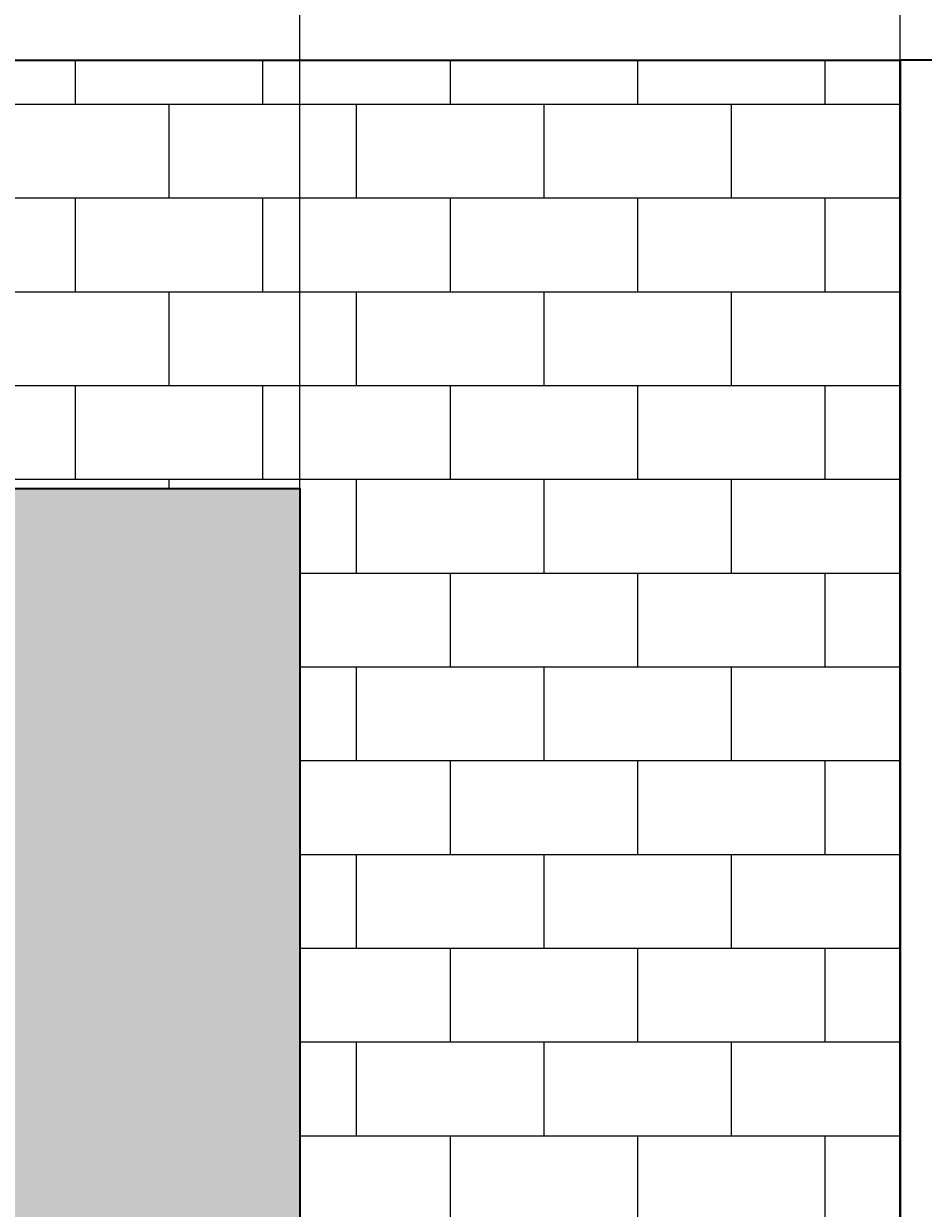
# Model space of a CAD drawing. Units: inches. Extents: x -13 to 809, y 112 to 656.
# Tile 52 of 55: x 521 to 593, y 467 to 561. Entities that reach past the tile are written whole.
import ezdxf

# ---------------------------------------------------------------- set-up
doc = ezdxf.new("R2010")
doc.units = ezdxf.units.IN
doc.header["$MEASUREMENT"] = 0
for name, color, linetype, lineweight in [('A-ANNO-DIMS', 2, 'Continuous', 18), ('A-ELEV', 7, 'Continuous', 35), ('A-ELEV-PATT', 8, 'Continuous', 13)]:
    doc.layers.add(name, color=color, linetype=linetype, lineweight=lineweight)
doc.styles.get("Standard").update_dxf_attribs({"font": 'arial.ttf'})
doc.dimstyles.get("Standard").update_dxf_attribs({"dimtxt": 0.625, "dimasz": 0.18, "dimexe": 0.18, "dimexo": 0.0625, "dimgap": 0.09, "dimtad": 0, "dimtih": 1, "dimtoh": 1, "dimdec": 4, "dimzin": 0, "dimdsep": 46, "dimlunit": 4, "dimtxsty": 'Standard', "dimcen": 0.09, "dimadec": 0, "dimazin": 0, "dimtfac": 1, "dimtdec": 4, "dimtofl": 0, "dimtmove": 0, "dimatfit": 3, "dimfxl": 1, "dimtolj": 1, "dimtzin": 0, "dimarcsym": 0})

# ---------------------------------------------------------------- blocks, each defined once
blk = doc.blocks.new('*D27')
at = {"layer": 'A-ANNO-DIMS', "color": 0, "lineweight": -2, "transparency": 16777216}
for p, q in [((471.1, 470.939), (471.1, 655.963)), ((471.28, 655.783), (505.889, 655.783)), ((542.782, 655.783), (508.173, 655.783)), ((542.962, 524.343), (542.962, 655.963))]:
    blk.add_line(p, q, dxfattribs=at)
at = {"layer": 'A-ANNO-DIMS', "color": 0, "transparency": 16777216}
for points in [[(471.28, 655.813), (471.28, 655.753), (471.1, 655.783)], [(542.782, 655.813), (542.782, 655.753), (542.962, 655.783)]]:
    blk.add_solid(points, dxfattribs=at)
at = {"layer": 'Defpoints', "color": 0, "transparency": 16777216}
for p in [(542.962, 655.783), (542.962, 524.281), (471.1, 470.877)]:
    blk.add_point(p, dxfattribs=at)
at = {"layer": 'A-ANNO-DIMS', "color": 0, "transparency": 16777216, "insert": (507.031, 655.783), "char_height": 0.625, "attachment_point": 5}
blk.add_mtext('\\A1;71.86', dxfattribs=at)
blk = doc.blocks.new('*D28')
at = {"layer": 'A-ANNO-DIMS', "color": 0, "lineweight": -2, "transparency": 16777216}
for p, q in [((542.962, 524.343), (542.962, 655.963)), ((543.142, 655.783), (565.825, 655.783)), ((590.828, 655.783), (568.144, 655.783)), ((591.008, 558.582), (591.008, 655.963))]:
    blk.add_line(p, q, dxfattribs=at)
at = {"layer": 'A-ANNO-DIMS', "color": 0, "transparency": 16777216}
for points in [[(543.142, 655.813), (543.142, 655.753), (542.962, 655.783)], [(590.828, 655.813), (590.828, 655.753), (591.008, 655.783)]]:
    blk.add_solid(points, dxfattribs=at)
at = {"layer": 'Defpoints', "color": 0, "transparency": 16777216}
for p in [(591.008, 655.783), (591.008, 558.52), (542.962, 524.281)]:
    blk.add_point(p, dxfattribs=at)
at = {"layer": 'A-ANNO-DIMS', "color": 0, "transparency": 16777216, "insert": (566.985, 655.783), "char_height": 0.625, "attachment_point": 5}
blk.add_mtext('\\A1;48.05', dxfattribs=at)
blk = doc.blocks.new('*D29')
at = {"layer": 'A-ANNO-DIMS', "color": 0, "lineweight": -2, "transparency": 16777216}
for p, q in [((591.008, 558.582), (591.008, 655.963)), ((591.188, 655.783), (605.472, 655.783)), ((620.828, 655.783), (606.544, 655.783)), ((621.008, 617.845), (621.008, 655.963))]:
    blk.add_line(p, q, dxfattribs=at)
at = {"layer": 'A-ANNO-DIMS', "color": 0, "transparency": 16777216}
for points in [[(591.188, 655.813), (591.188, 655.753), (591.008, 655.783)], [(620.828, 655.813), (620.828, 655.753), (621.008, 655.783)]]:
    blk.add_solid(points, dxfattribs=at)
at = {"layer": 'Defpoints', "color": 0, "transparency": 16777216}
for p in [(621.008, 655.783), (621.008, 617.783), (591.008, 558.52)]:
    blk.add_point(p, dxfattribs=at)
at = {"layer": 'A-ANNO-DIMS', "color": 0, "transparency": 16777216, "insert": (606.008, 655.783), "char_height": 0.625, "attachment_point": 5}
blk.add_mtext('\\A1;30', dxfattribs=at)

msp = doc.modelspace()

# ---------------------------------------------------------------- hatches: boundary and pattern name
at = {"layer": 'A-ELEV-PATT'}
h = msp.add_hatch(dxfattribs=at)
h.set_pattern_fill('BRICK', color=256, scale=30)
h.paths.add_polyline_path([(591.008, 558.5199), (341.4072, 558.5199), (341.4072, 524.281), (542.9617, 524.281), (542.9617, 288.4508), (341.4072, 288.4508), (341.4072, 250.8429), (591.008, 250.8429)])
h = msp.add_hatch(dxfattribs=at)
h.set_pattern_fill('CROSS', color=256, scale=9.7)
h.paths.add_polyline_path([(542.9617, 524.281), (442.1845, 524.281), (442.1845, 288.4508), (542.9617, 288.4508)])
h.paths.add_polyline_path([(471.0998, 470.8765), (471.0998, 498.1452), (510.462, 498.1452), (510.462, 470.8765)], flags=16)
h.paths.add_polyline_path([(473.0998, 472.8765), (473.0998, 496.1452), (508.462, 496.1452), (508.462, 472.8765)], flags=0)
h.paths.add_polyline_path([(471.0998, 442.128), (510.462, 442.128), (510.462, 414.8594), (471.0998, 414.8594)], flags=16)
h.paths.add_polyline_path([(473.0998, 440.128), (508.462, 440.128), (508.462, 416.8594), (473.0998, 416.8594)], flags=0)
h.paths.add_polyline_path([(471.0998, 385.2491), (510.462, 385.2491), (510.462, 357.9804), (471.0998, 357.9804)], flags=16)
h.paths.add_polyline_path([(473.0998, 383.2491), (508.462, 383.2491), (508.462, 359.9804), (473.0998, 359.9804)], flags=0)
h.paths.add_polyline_path([(471.0998, 340.4353), (510.462, 340.4353), (510.462, 313.1667), (471.0998, 313.1667)], flags=16)
h.paths.add_polyline_path([(473.0998, 338.4353), (508.462, 338.4353), (508.462, 315.1667), (473.0998, 315.1667)], flags=0)

# ---------------------------------------------------------------- linework, layer by layer
at = {"layer": 'A-ELEV'}
for p in [(341.4072, 558.5199), (591.008, 209.8635), (644.6221, 558.5199)]:
    msp.add_line(p, (591.008, 558.5199), dxfattribs=at)
for points in [[(341.4072, 558.5199), (591.008, 558.5199), (591.008, 250.8429), (341.4072, 250.8429)], [(341.4072, 524.281), (542.9617, 524.281), (542.9617, 288.4508), (341.4072, 288.4508)]]:
    msp.add_lwpolyline(points, close=True, dxfattribs=at)

# ---------------------------------------------------------------- dimensions: what is measured, and where the dimension line sits
at = {"layer": 'A-ANNO-DIMS'}
for base, p1, p2, override, picture, middle in [((542.9617, 655.7828), (471.0998, 470.8765), (542.9617, 524.281), {"dimdec": 2, "dimlfac": 1, "dimrnd": 0, "dimzin": 0, "dimdsep": 46, "dimlunit": 2}, '*D27', (507.0308, 655.7828)), ((591.008, 655.7828), (542.9617, 524.281), (591.008, 558.5199), {"dimdec": 2, "dimlfac": 1, "dimrnd": 0, "dimzin": 0, "dimdsep": 46, "dimlunit": 2}, '*D28', (566.9849, 655.7828)), ((621.008, 655.7828), (591.008, 558.5199), (621.008, 617.7828), {"dimdec": 0, "dimlfac": 1, "dimrnd": 0, "dimzin": 0, "dimdsep": 46, "dimlunit": 2}, '*D29', (606.008, 655.7828))]:
    dim = msp.add_linear_dim(base=base, p1=p1, p2=p2, dimstyle='Standard', override=override, dxfattribs=at)
    dim.commit()
    dim.dimension.update_dxf_attribs({"geometry": picture, "text_midpoint": middle})

doc.saveas('drawing.dxf')
